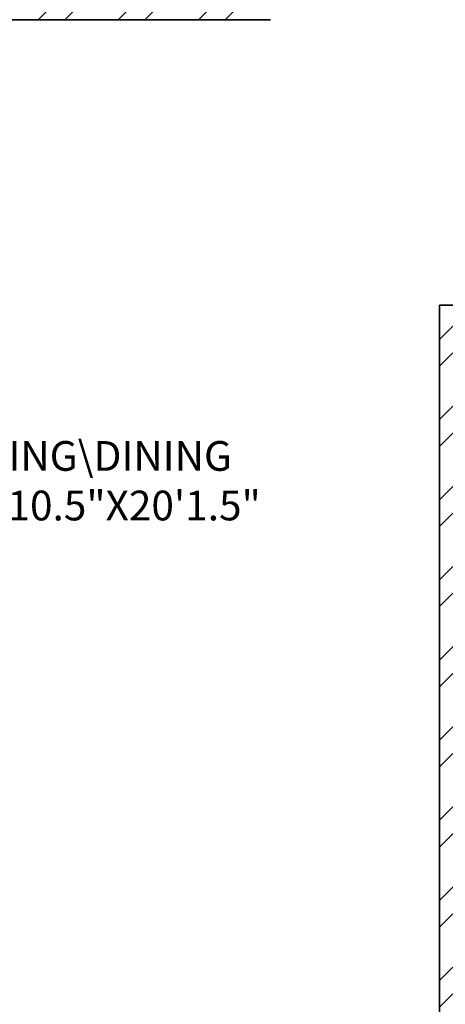
# Model space of a CAD drawing. Units: inches. Extents: x 2120 to 4013, y 1390 to 3019.
# Tile 38 of 59: x 2789 to 2861, y 2048 to 2213. Entities that reach past the tile are written whole.
import ezdxf

# ---------------------------------------------------------------- set-up
doc = ezdxf.new("R2010")
doc.units = ezdxf.units.IN
for name, color, linetype, lineweight in [('A-AREA-IDEN', 7, 'Continuous', 18), ('A-WALL', 7, 'Continuous', 35), ('A-WALL-PATT', 252, 'Continuous', 13)]:
    doc.layers.add(name, color=color, linetype=linetype, lineweight=lineweight)
doc.styles.get("Standard").update_dxf_attribs({"font": 'arial.ttf'})

msp = doc.modelspace()

# ---------------------------------------------------------------- hatches: boundary and pattern name
at = {"layer": 'A-WALL-PATT'}
h = msp.add_hatch(dxfattribs=at)
h.set_pattern_fill('ANSI32', color=256)
h.paths.add_polyline_path([(2271.7331, 2343.531), (2283.3788, 2343.531), (2283.3788, 2348.031), (2283.3788, 2352.5306), (2262.7331, 2352.5306), (2262.7331, 2182.638), (2267.2331, 2182.638), (2271.7331, 2182.638), (2271.7331, 2219.031), (2391.7331, 2219.031), (2391.7331, 2214.189), (2393.9831, 2214.189), (2396.2331, 2214.189), (2396.2331, 2219.031), (2420.2331, 2219.031), (2420.2331, 2225.7535), (2417.2197, 2225.7535), (2415.7331, 2225.7535), (2415.7331, 2223.5306), (2271.7331, 2223.5306)])
h.paths.add_polyline_path([(2380.0942, 2352.5306), (2343.3788, 2352.5306), (2343.3788, 2343.531), (2363.2331, 2343.531), (2363.2331, 2288.8489), (2365.4831, 2288.8489), (2367.7331, 2288.8489), (2367.7331, 2343.531), (2380.0942, 2343.531)], flags=17)
h.paths.add_polyline_path([(2432.4339, 2352.5306), (2404.0943, 2352.5306), (2404.0943, 2343.531), (2415.7331, 2343.531), (2415.7331, 2264.0306), (2367.7331, 2264.0306), (2367.7331, 2266.4872), (2363.2331, 2266.4872), (2363.2331, 2259.531), (2367.7331, 2259.531), (2415.7331, 2259.531), (2415.7331, 2255.0658), (2420.2331, 2255.0658), (2420.2331, 2259.531), (2424.5717, 2259.531), (2424.5717, 2261.781), (2424.5717, 2264.0306), (2420.2331, 2264.0306), (2420.2331, 2343.531), (2432.4339, 2343.531)])
h.paths.add_polyline_path([(2508.9115, 2352.5306), (2456.4339, 2352.5306), (2456.4339, 2343.531), (2468.2331, 2343.531), (2468.2331, 2264.0306), (2448.0487, 2264.0306), (2448.0487, 2259.531), (2468.2331, 2259.531), (2468.2331, 2255.5496), (2472.7331, 2255.5496), (2472.7331, 2343.531), (2508.9115, 2343.531)])
h.paths.add_polyline_path([(2637.7331, 2352.5306), (2544.9116, 2352.5306), (2544.9116, 2343.531), (2589.7331, 2343.531), (2633.2331, 2343.531), (2637.7331, 2343.531)])
h.paths.add_polyline_path([(2594.2331, 2343.5306), (2589.7331, 2343.5306), (2589.7331, 2259.5306), (2589.7331, 2252.4915), (2591.9831, 2252.4915), (2594.2331, 2252.4915)])
h.paths.add_polyline_path([(2637.7331, 2223.5306), (2594.2331, 2223.5306), (2594.2331, 2230.1988), (2591.9831, 2230.1988), (2589.7331, 2230.1988), (2589.7331, 2223.5306), (2472.7331, 2223.5306), (2468.2331, 2223.5306), (2468.2331, 2219.031), (2628.7331, 2219.031), (2628.7331, 2138.031), (2637.7331, 2138.031)])
h.paths.add_polyline_path([(3822.6535, 2458.4402), (3874.9468, 2458.4402), (3874.9468, 2476.9866), (3822.6535, 2476.9866)], flags=9)
h.paths.add_polyline_path([(3834.6921, 2781.8174), (3935.9206, 2781.8174), (3935.9206, 2800.3638), (3834.6921, 2800.3638)], flags=9)
h.paths.add_polyline_path([(3832.2843, 2837.9683), (3884.5776, 2837.9683), (3884.5776, 2856.5146), (3832.2843, 2856.5146)], flags=9)
h.paths.add_polyline_path([(3830.9388, 2861.4782), (3956.8958, 2861.4782), (3956.8958, 2880.0245), (3830.9388, 2880.0245)], flags=9)
h.paths.add_polyline_path([(3870.6966, 2352.5752), (3887.9272, 2352.5752), (3887.9272, 2377.3037), (3870.6966, 2377.3037)], flags=9)
h.paths.add_polyline_path([(3289.2701, 2413.161), (3435.2223, 2413.161), (3435.2223, 2450.2538), (3289.2701, 2450.2538)], flags=9)
h.paths.add_polyline_path([(2487.6944, 2414.3601), (2637.8335, 2414.3601), (2637.8335, 2451.4528), (2487.6944, 2451.4528)], flags=9)
h.paths.add_polyline_path([(2567.3724, 1457.9199), (2815.296, 1457.9199), (2815.296, 1495.0127), (2567.3724, 1495.0127)], flags=9)
h.paths.add_polyline_path([(2655.3825, 2093.2363), (2685.9555, 2093.2363), (2685.9555, 2111.8937), (2655.3825, 2111.8937)], flags=9)
h.paths.add_polyline_path([(2543.9218, 1550.6671), (2587.8406, 1550.6671), (2587.8406, 1569.3244), (2543.9218, 1569.3244)], flags=9)
h.paths.add_polyline_path([(2905.1384, 1543.8113), (2949.0572, 1543.8113), (2949.0572, 1562.4686), (2905.1384, 1562.4686)], flags=9)
h.paths.add_polyline_path([(2736.4118, 1702.4736), (2784.2153, 1702.4736), (2784.2153, 1721.1309), (2736.4118, 1721.1309)], flags=9)
h.paths.add_polyline_path([(2912.8666, 1710.4168), (2951.707, 1710.4168), (2951.707, 1729.0741), (2912.8666, 1729.0741)], flags=9)
h.paths.add_polyline_path([(2923.5785, 1763.5038), (2959.7279, 1763.5038), (2959.7279, 1782.1611), (2923.5785, 1782.1611)], flags=9)
h.paths.add_polyline_path([(2925.2114, 1809.6137), (2967.1861, 1809.6137), (2967.1861, 1828.271), (2925.2114, 1828.271)], flags=9)
h.paths.add_polyline_path([(2996.2711, 1878.9003), (2996.2711, 1913.109), (2977.6138, 1913.109), (2977.6138, 1878.9003)], flags=9)
h.paths.add_polyline_path([(2883.0859, 1895.7192), (2927.1855, 1895.7192), (2927.1855, 1914.3766), (2883.0859, 1914.3766)], flags=9)
h.paths.add_polyline_path([(2787.3924, 1810.8013), (2841.0213, 1810.8013), (2841.0213, 1829.4587), (2787.3924, 1829.4587)], flags=9)
h.paths.add_polyline_path([(2775.6399, 2101.7395), (2829.2689, 2101.7395), (2829.2689, 2120.3968), (2775.6399, 2120.3968)], flags=9)
h.paths.add_polyline_path([(2913.0263, 2075.817), (2951.8667, 2075.817), (2951.8667, 2094.4744), (2913.0263, 2094.4744)], flags=9)
h.paths.add_polyline_path([(2929.966, 2133.3669), (2966.1154, 2133.3669), (2966.1154, 2152.0243), (2929.966, 2152.0243)], flags=9)
h.paths.add_polyline_path([(2932.7502, 2182.6088), (2968.8996, 2182.6088), (2968.8996, 2201.2662), (2932.7502, 2201.2662)], flags=9)
h.paths.add_polyline_path([(2996.0681, 2266.3173), (2996.0681, 2300.5261), (2977.4108, 2300.5261), (2977.4108, 2266.3173)], flags=9)
h.paths.add_polyline_path([(2885.1039, 2279.2186), (2929.2035, 2279.2186), (2929.2035, 2297.8759), (2885.1039, 2297.8759)], flags=9)
h.paths.add_polyline_path([(2735.7042, 2218.3197), (2783.5078, 2218.3197), (2783.5078, 2236.9771), (2735.7042, 2236.9771)], flags=9)
h.paths.add_polyline_path([(2635.6049, 2044.0085), (2648.9678, 2044.0085), (2648.9678, 2054.312), (2635.6049, 2054.312)], flags=9)
h.paths.add_polyline_path([(2714.0148, 1923.0473), (2727.3777, 1923.0473), (2727.3777, 1933.3508), (2714.0148, 1933.3508)], flags=9)
h.paths.add_polyline_path([(2709.0345, 1988.1628), (2722.3974, 1988.1628), (2722.3974, 1998.4663), (2709.0345, 1998.4663)], flags=9)
h.paths.add_polyline_path([(2592.8935, 1962.1763), (2606.2564, 1962.1763), (2606.2564, 1972.4799), (2592.8935, 1972.4799)], flags=9)
h.paths.add_polyline_path([(2618.3996, 1985.9724), (2644.1942, 1985.9724), (2644.1942, 1996.2759), (2618.3996, 1996.2759)], flags=9)
h.paths.add_polyline_path([(2601.279, 1920.5869), (2614.6419, 1920.5869), (2614.6419, 1930.8904), (2601.279, 1930.8904)], flags=9)
h.paths.add_polyline_path([(2692.3278, 1932.7645), (2704.5311, 1932.7645), (2704.5311, 1943.0681), (2692.3278, 1943.0681)], flags=9)
h.paths.add_polyline_path([(2311.122, 1672.7318), (2355.0408, 1672.7318), (2355.0408, 1691.3892), (2311.122, 1691.3892)], flags=9)
h.paths.add_polyline_path([(2456.2551, 1632.3198), (2492.4796, 1632.3198), (2492.4796, 1650.9772), (2456.2551, 1650.9772)], flags=9)
h.paths.add_polyline_path([(2401.0766, 1631.4793), (2437.301, 1631.4793), (2437.301, 1650.1367), (2401.0766, 1650.1367)], flags=9)
h.paths.add_polyline_path([(2546.7054, 1700.9235), (2594.509, 1700.9235), (2594.509, 1719.5809), (2546.7054, 1719.5809)], flags=9)
h.paths.add_polyline_path([(2445.4866, 1766.9937), (2497.5261, 1766.9937), (2497.5261, 1785.651), (2445.4866, 1785.651)], flags=9)
h.paths.add_polyline_path([(2287.9992, 1739.7675), (2326.8396, 1739.7675), (2326.8396, 1758.4248), (2287.9992, 1758.4248)], flags=9)
h.paths.add_polyline_path([(2458.5279, 1924.7607), (2510.5675, 1924.7607), (2510.5675, 1943.4181), (2458.5279, 1943.4181)], flags=9)
h.paths.add_polyline_path([(2309.2811, 1902.7642), (2345.4305, 1902.7642), (2345.4305, 1921.4215), (2309.2811, 1921.4215)], flags=9)
h.paths.add_polyline_path([(2490.7554, 2018.9392), (2530.7896, 2018.9392), (2530.7896, 2037.5965), (2490.7554, 2037.5965)], flags=9)
h.paths.add_polyline_path([(2402.143, 2024.7393), (2438.5414, 2024.7393), (2438.5414, 2043.3966), (2402.143, 2043.3966)], flags=9)
h.paths.add_polyline_path([(2287.856, 1931.7926), (2326.6964, 1931.7926), (2326.6964, 1950.4499), (2287.856, 1950.4499)], flags=9)
h.paths.add_polyline_path([(2281.7979, 2193.5771), (2320.6383, 2193.5771), (2320.6383, 2212.2344), (2281.7979, 2212.2344)], flags=25)
h.paths.add_polyline_path([(2484.0754, 2093.892), (2536.115, 2093.892), (2536.115, 2112.5494), (2484.0754, 2112.5494)], flags=9)
h.paths.add_polyline_path([(2624.7948, 2281.8639), (2624.7948, 2311.4137), (2606.1375, 2311.4137), (2606.1375, 2281.8639)], flags=9)
h.paths.add_polyline_path([(2507.5036, 2290.3639), (2541.934, 2290.3639), (2541.934, 2309.0212), (2507.5036, 2309.0212)], flags=9)
h.paths.add_polyline_path([(2423.1076, 2285.2202), (2459.332, 2285.2202), (2459.332, 2303.8776), (2423.1076, 2303.8776)], flags=9)
h.paths.add_polyline_path([(2374.5467, 2289.6272), (2410.7711, 2289.6272), (2410.7711, 2308.2846), (2374.5467, 2308.2846)], flags=25)
h.paths.add_polyline_path([(2277.4907, 2227.5651), (2316.3311, 2227.5651), (2316.3311, 2246.2224), (2277.4907, 2246.2224)], flags=25)
h.paths.add_polyline_path([(2655.3825, 2093.2367), (2685.9555, 2093.2367), (2685.9555, 2111.894), (2655.3825, 2111.894)], flags=9)
h.paths.add_polyline_path([(2543.9217, 1550.6674), (2587.8406, 1550.6674), (2587.8406, 1569.3247), (2543.9217, 1569.3247)], flags=9)
h.paths.add_polyline_path([(2905.1384, 1543.8116), (2949.0572, 1543.8116), (2949.0572, 1562.4689), (2905.1384, 1562.4689)], flags=9)
h.paths.add_polyline_path([(2736.4118, 1702.4739), (2784.2153, 1702.4739), (2784.2153, 1721.1312), (2736.4118, 1721.1312)], flags=9)
h.paths.add_polyline_path([(2912.8666, 1710.4171), (2951.707, 1710.4171), (2951.707, 1729.0744), (2912.8666, 1729.0744)], flags=9)
h.paths.add_polyline_path([(2923.5785, 1763.5041), (2959.7279, 1763.5041), (2959.7279, 1782.1614), (2923.5785, 1782.1614)], flags=9)
h.paths.add_polyline_path([(2925.2114, 1809.614), (2967.1861, 1809.614), (2967.1861, 1828.2713), (2925.2114, 1828.2713)], flags=9)
h.paths.add_polyline_path([(2996.2711, 1878.9006), (2996.2711, 1913.1094), (2977.6137, 1913.1094), (2977.6137, 1878.9006)], flags=9)
h.paths.add_polyline_path([(2883.0859, 1895.7195), (2927.1855, 1895.7195), (2927.1855, 1914.3769), (2883.0859, 1914.3769)], flags=9)
h.paths.add_polyline_path([(2787.3924, 1810.8016), (2841.0213, 1810.8016), (2841.0213, 1829.459), (2787.3924, 1829.459)], flags=9)
h.paths.add_polyline_path([(2775.6399, 2101.7398), (2829.2688, 2101.7398), (2829.2688, 2120.3971), (2775.6399, 2120.3971)], flags=9)
h.paths.add_polyline_path([(2913.0263, 2075.8173), (2951.8667, 2075.8173), (2951.8667, 2094.4747), (2913.0263, 2094.4747)], flags=9)
h.paths.add_polyline_path([(2929.966, 2133.3672), (2966.1154, 2133.3672), (2966.1154, 2152.0246), (2929.966, 2152.0246)], flags=9)
h.paths.add_polyline_path([(2932.7502, 2182.6091), (2968.8996, 2182.6091), (2968.8996, 2201.2665), (2932.7502, 2201.2665)], flags=9)
h.paths.add_polyline_path([(2996.0681, 2266.3176), (2996.0681, 2300.5264), (2977.4108, 2300.5264), (2977.4108, 2266.3176)], flags=9)
h.paths.add_polyline_path([(2885.1039, 2279.2189), (2929.2035, 2279.2189), (2929.2035, 2297.8762), (2885.1039, 2297.8762)], flags=9)
h.paths.add_polyline_path([(2735.7042, 2218.32), (2783.5078, 2218.32), (2783.5078, 2236.9774), (2735.7042, 2236.9774)], flags=9)
h.paths.add_polyline_path([(2635.6048, 2044.0088), (2648.9677, 2044.0088), (2648.9677, 2054.3123), (2635.6048, 2054.3123)], flags=9)
h.paths.add_polyline_path([(2714.0148, 1923.0476), (2727.3777, 1923.0476), (2727.3777, 1933.3511), (2714.0148, 1933.3511)], flags=9)
h.paths.add_polyline_path([(2709.0345, 1988.1631), (2722.3974, 1988.1631), (2722.3974, 1998.4666), (2709.0345, 1998.4666)], flags=9)
h.paths.add_polyline_path([(2592.8935, 1962.1766), (2606.2564, 1962.1766), (2606.2564, 1972.4802), (2592.8935, 1972.4802)], flags=9)
h.paths.add_polyline_path([(2618.3995, 1985.9727), (2644.1942, 1985.9727), (2644.1942, 1996.2762), (2618.3995, 1996.2762)], flags=9)
h.paths.add_polyline_path([(2601.279, 1920.5872), (2614.6419, 1920.5872), (2614.6419, 1930.8908), (2601.279, 1930.8908)], flags=9)
h.paths.add_polyline_path([(2692.3278, 1932.7648), (2704.5311, 1932.7648), (2704.5311, 1943.0684), (2692.3278, 1943.0684)], flags=9)
h.paths.add_polyline_path([(2311.122, 1672.7321), (2355.0408, 1672.7321), (2355.0408, 1691.3895), (2311.122, 1691.3895)], flags=9)
h.paths.add_polyline_path([(2456.2551, 1632.3201), (2492.4795, 1632.3201), (2492.4795, 1650.9775), (2456.2551, 1650.9775)], flags=9)
h.paths.add_polyline_path([(2401.0766, 1631.4796), (2437.301, 1631.4796), (2437.301, 1650.137), (2401.0766, 1650.137)], flags=9)
h.paths.add_polyline_path([(2546.7054, 1700.9238), (2594.509, 1700.9238), (2594.509, 1719.5812), (2546.7054, 1719.5812)], flags=9)
h.paths.add_polyline_path([(2445.4866, 1766.994), (2497.5261, 1766.994), (2497.5261, 1785.6513), (2445.4866, 1785.6513)], flags=9)
h.paths.add_polyline_path([(2287.9992, 1739.7678), (2326.8396, 1739.7678), (2326.8396, 1758.4251), (2287.9992, 1758.4251)], flags=9)
h.paths.add_polyline_path([(2458.5279, 1924.7611), (2510.5675, 1924.7611), (2510.5675, 1943.4184), (2458.5279, 1943.4184)], flags=9)
h.paths.add_polyline_path([(2309.2811, 1902.7645), (2345.4305, 1902.7645), (2345.4305, 1921.4218), (2309.2811, 1921.4218)], flags=9)
h.paths.add_polyline_path([(2490.7554, 2018.9395), (2530.7895, 2018.9395), (2530.7895, 2037.5968), (2490.7554, 2037.5968)], flags=9)
h.paths.add_polyline_path([(2402.143, 2024.7396), (2438.5413, 2024.7396), (2438.5413, 2043.3969), (2402.143, 2043.3969)], flags=9)
h.paths.add_polyline_path([(2287.856, 1931.7929), (2326.6964, 1931.7929), (2326.6964, 1950.4502), (2287.856, 1950.4502)], flags=9)
h.paths.add_polyline_path([(2281.7979, 2193.5774), (2320.6383, 2193.5774), (2320.6383, 2212.2347), (2281.7979, 2212.2347)], flags=25)
h.paths.add_polyline_path([(2484.0754, 2093.8924), (2536.115, 2093.8924), (2536.115, 2112.5497), (2484.0754, 2112.5497)], flags=9)
h.paths.add_polyline_path([(2624.7948, 2281.8642), (2624.7948, 2311.414), (2606.1374, 2311.414), (2606.1374, 2281.8642)], flags=9)
h.paths.add_polyline_path([(2507.5035, 2290.3642), (2541.934, 2290.3642), (2541.934, 2309.0215), (2507.5035, 2309.0215)], flags=9)
h.paths.add_polyline_path([(2423.1075, 2285.2205), (2459.332, 2285.2205), (2459.332, 2303.8779), (2423.1075, 2303.8779)], flags=9)
h.paths.add_polyline_path([(2374.5467, 2289.6275), (2410.7711, 2289.6275), (2410.7711, 2308.2849), (2374.5467, 2308.2849)], flags=25)
h.paths.add_polyline_path([(2277.4907, 2227.5654), (2316.3311, 2227.5654), (2316.3311, 2246.2227), (2277.4907, 2246.2227)], flags=25)
h = msp.add_hatch(dxfattribs=at)
h.set_pattern_fill('ANSI32', color=256)
h.paths.add_polyline_path([(2271.7331, 1980.389), (2262.7331, 1980.389), (2262.7331, 1912.8434), (2267.2331, 1912.8434), (2271.7331, 1912.8434), (2271.7331, 1922.531), (2351.2331, 1922.531), (2351.2331, 1901.4728), (2355.7331, 1901.4728), (2355.7331, 1922.531), (2357.9815, 1922.531), (2357.9815, 1926.5306), (2271.7331, 1926.5306)])
h.paths.add_polyline_path([(2589.2331, 1949.1622), (2584.7331, 1949.1622), (2580.2331, 1949.1622), (2580.2331, 1874.5306), (2355.7331, 1874.5306), (2355.7331, 1880.1922), (2351.2331, 1880.1922), (2351.2331, 1874.5306), (2271.7331, 1874.5306), (2271.7331, 1888.8431), (2262.7331, 1888.8431), (2262.7331, 1842.2909), (2267.2331, 1842.2909), (2271.7331, 1842.2909), (2271.7331, 1865.531), (2415.7331, 1865.531), (2415.7331, 1779.7286), (2420.2331, 1779.7286), (2420.2331, 1865.531), (2589.2331, 1865.531)])
h.paths.add_polyline_path([(2271.7331, 1782.2906), (2262.7331, 1782.2906), (2262.7331, 1711.4639), (2267.2331, 1711.4639), (2271.7331, 1711.4639), (2271.7331, 1738.031), (2420.2331, 1738.031), (2420.2331, 1742.531), (2420.2331, 1747.3376), (2417.9831, 1747.3376), (2415.7331, 1747.3376), (2415.7331, 1742.5306), (2271.7331, 1742.5306)])
h.paths.add_polyline_path([(2271.7331, 1627.031), (2362.3957, 1627.031), (2362.3957, 1629.281), (2362.3957, 1631.5306), (2271.7331, 1631.5306), (2271.7331, 1675.4636), (2262.7331, 1675.4636), (2262.7331, 1581.531), (2405.3032, 1581.531), (2405.3032, 1586.031), (2405.3032, 1590.5306), (2396.2331, 1590.5306), (2396.2331, 1691.4513), (2418.7206, 1691.4513), (2418.7206, 1695.951), (2396.2331, 1695.951), (2391.7331, 1695.951), (2391.7331, 1631.5306), (2386.7425, 1631.5306), (2386.7425, 1629.2806), (2386.7425, 1627.031), (2391.7331, 1627.031), (2391.7331, 1586.1709), (2271.7331, 1586.1709)])
h.paths.add_polyline_path([(2459.6703, 1590.5306), (2429.3032, 1590.5306), (2429.3032, 1581.531), (2459.6703, 1581.531), (2459.6703, 1586.031)])
h.paths.add_polyline_path([(2501.2331, 1590.531), (2501.2331, 1665.0195), (2498.9831, 1665.0195), (2496.7331, 1665.0195), (2496.7331, 1590.5306), (2483.8201, 1590.5306), (2483.8201, 1590.1579), (2483.6704, 1590.1579), (2483.6704, 1581.531), (2505.0196, 1581.531), (2505.0196, 1583.781), (2505.0196, 1586.0306), (2501.2331, 1586.0306)])
h.paths.add_polyline_path([(2544.1361, 1583.781), (2544.1361, 1586.0306), (2527.1368, 1586.0306), (2527.1368, 1583.7806), (2527.1368, 1581.531), (2544.1361, 1581.531)])
h.paths.add_polyline_path([(3822.6535, 2458.4402), (3874.9468, 2458.4402), (3874.9468, 2476.9866), (3822.6535, 2476.9866)], flags=9)
h.paths.add_polyline_path([(3834.6921, 2781.8174), (3935.9206, 2781.8174), (3935.9206, 2800.3638), (3834.6921, 2800.3638)], flags=9)
h.paths.add_polyline_path([(3832.2843, 2837.9683), (3884.5776, 2837.9683), (3884.5776, 2856.5146), (3832.2843, 2856.5146)], flags=9)
h.paths.add_polyline_path([(3830.9388, 2861.4782), (3956.8958, 2861.4782), (3956.8958, 2880.0245), (3830.9388, 2880.0245)], flags=9)
h.paths.add_polyline_path([(3870.6966, 2352.5752), (3887.9272, 2352.5752), (3887.9272, 2377.3037), (3870.6966, 2377.3037)], flags=9)
h.paths.add_polyline_path([(3289.2701, 2413.161), (3435.2223, 2413.161), (3435.2223, 2450.2538), (3289.2701, 2450.2538)], flags=9)
h.paths.add_polyline_path([(2487.6944, 2414.3601), (2637.8335, 2414.3601), (2637.8335, 2451.4528), (2487.6944, 2451.4528)], flags=9)
h.paths.add_polyline_path([(2567.3724, 1457.9199), (2815.296, 1457.9199), (2815.296, 1495.0127), (2567.3724, 1495.0127)], flags=9)
h.paths.add_polyline_path([(2655.3825, 2093.2363), (2685.9555, 2093.2363), (2685.9555, 2111.8937), (2655.3825, 2111.8937)], flags=9)
h.paths.add_polyline_path([(2543.9218, 1550.6671), (2587.8406, 1550.6671), (2587.8406, 1569.3244), (2543.9218, 1569.3244)], flags=9)
h.paths.add_polyline_path([(2905.1384, 1543.8113), (2949.0572, 1543.8113), (2949.0572, 1562.4686), (2905.1384, 1562.4686)], flags=9)
h.paths.add_polyline_path([(2736.4118, 1702.4736), (2784.2153, 1702.4736), (2784.2153, 1721.1309), (2736.4118, 1721.1309)], flags=9)
h.paths.add_polyline_path([(2912.8666, 1710.4168), (2951.707, 1710.4168), (2951.707, 1729.0741), (2912.8666, 1729.0741)], flags=9)
h.paths.add_polyline_path([(2923.5785, 1763.5038), (2959.7279, 1763.5038), (2959.7279, 1782.1611), (2923.5785, 1782.1611)], flags=9)
h.paths.add_polyline_path([(2925.2114, 1809.6137), (2967.1861, 1809.6137), (2967.1861, 1828.271), (2925.2114, 1828.271)], flags=9)
h.paths.add_polyline_path([(2996.2711, 1878.9003), (2996.2711, 1913.109), (2977.6138, 1913.109), (2977.6138, 1878.9003)], flags=9)
h.paths.add_polyline_path([(2883.0859, 1895.7192), (2927.1855, 1895.7192), (2927.1855, 1914.3766), (2883.0859, 1914.3766)], flags=9)
h.paths.add_polyline_path([(2787.3924, 1810.8013), (2841.0213, 1810.8013), (2841.0213, 1829.4587), (2787.3924, 1829.4587)], flags=9)
h.paths.add_polyline_path([(2775.6399, 2101.7395), (2829.2689, 2101.7395), (2829.2689, 2120.3968), (2775.6399, 2120.3968)], flags=9)
h.paths.add_polyline_path([(2913.0263, 2075.817), (2951.8667, 2075.817), (2951.8667, 2094.4744), (2913.0263, 2094.4744)], flags=9)
h.paths.add_polyline_path([(2929.966, 2133.3669), (2966.1154, 2133.3669), (2966.1154, 2152.0243), (2929.966, 2152.0243)], flags=9)
h.paths.add_polyline_path([(2932.7502, 2182.6088), (2968.8996, 2182.6088), (2968.8996, 2201.2662), (2932.7502, 2201.2662)], flags=9)
h.paths.add_polyline_path([(2996.0681, 2266.3173), (2996.0681, 2300.5261), (2977.4108, 2300.5261), (2977.4108, 2266.3173)], flags=9)
h.paths.add_polyline_path([(2885.1039, 2279.2186), (2929.2035, 2279.2186), (2929.2035, 2297.8759), (2885.1039, 2297.8759)], flags=9)
h.paths.add_polyline_path([(2735.7042, 2218.3197), (2783.5078, 2218.3197), (2783.5078, 2236.9771), (2735.7042, 2236.9771)], flags=9)
h.paths.add_polyline_path([(2635.6049, 2044.0085), (2648.9678, 2044.0085), (2648.9678, 2054.312), (2635.6049, 2054.312)], flags=9)
h.paths.add_polyline_path([(2714.0148, 1923.0473), (2727.3777, 1923.0473), (2727.3777, 1933.3508), (2714.0148, 1933.3508)], flags=9)
h.paths.add_polyline_path([(2709.0345, 1988.1628), (2722.3974, 1988.1628), (2722.3974, 1998.4663), (2709.0345, 1998.4663)], flags=9)
h.paths.add_polyline_path([(2592.8935, 1962.1763), (2606.2564, 1962.1763), (2606.2564, 1972.4799), (2592.8935, 1972.4799)], flags=9)
h.paths.add_polyline_path([(2618.3996, 1985.9724), (2644.1942, 1985.9724), (2644.1942, 1996.2759), (2618.3996, 1996.2759)], flags=9)
h.paths.add_polyline_path([(2601.279, 1920.5869), (2614.6419, 1920.5869), (2614.6419, 1930.8904), (2601.279, 1930.8904)], flags=9)
h.paths.add_polyline_path([(2692.3278, 1932.7645), (2704.5311, 1932.7645), (2704.5311, 1943.0681), (2692.3278, 1943.0681)], flags=9)
h.paths.add_polyline_path([(2311.122, 1672.7318), (2355.0408, 1672.7318), (2355.0408, 1691.3892), (2311.122, 1691.3892)], flags=25)
h.paths.add_polyline_path([(2456.2551, 1632.3198), (2492.4796, 1632.3198), (2492.4796, 1650.9772), (2456.2551, 1650.9772)], flags=9)
h.paths.add_polyline_path([(2401.0766, 1631.4793), (2437.301, 1631.4793), (2437.301, 1650.1367), (2401.0766, 1650.1367)], flags=9)
h.paths.add_polyline_path([(2546.7054, 1700.9235), (2594.509, 1700.9235), (2594.509, 1719.5809), (2546.7054, 1719.5809)], flags=9)
h.paths.add_polyline_path([(2445.4866, 1766.9937), (2497.5261, 1766.9937), (2497.5261, 1785.651), (2445.4866, 1785.651)], flags=9)
h.paths.add_polyline_path([(2287.9992, 1739.7675), (2326.8396, 1739.7675), (2326.8396, 1758.4248), (2287.9992, 1758.4248)], flags=24)
h.paths.add_polyline_path([(2458.5279, 1924.7607), (2510.5675, 1924.7607), (2510.5675, 1943.4181), (2458.5279, 1943.4181)], flags=25)
h.paths.add_polyline_path([(2309.2811, 1902.7642), (2345.4305, 1902.7642), (2345.4305, 1921.4215), (2309.2811, 1921.4215)], flags=25)
h.paths.add_polyline_path([(2490.7554, 2018.9392), (2530.7896, 2018.9392), (2530.7896, 2037.5965), (2490.7554, 2037.5965)], flags=9)
h.paths.add_polyline_path([(2402.143, 2024.7393), (2438.5414, 2024.7393), (2438.5414, 2043.3966), (2402.143, 2043.3966)], flags=9)
h.paths.add_polyline_path([(2287.856, 1931.7926), (2326.6964, 1931.7926), (2326.6964, 1950.4499), (2287.856, 1950.4499)], flags=25)
h.paths.add_polyline_path([(2281.7979, 2193.5771), (2320.6383, 2193.5771), (2320.6383, 2212.2344), (2281.7979, 2212.2344)], flags=9)
h.paths.add_polyline_path([(2484.0754, 2093.892), (2536.115, 2093.892), (2536.115, 2112.5494), (2484.0754, 2112.5494)], flags=9)
h.paths.add_polyline_path([(2624.7948, 2281.8639), (2624.7948, 2311.4137), (2606.1375, 2311.4137), (2606.1375, 2281.8639)], flags=9)
h.paths.add_polyline_path([(2507.5036, 2290.3639), (2541.934, 2290.3639), (2541.934, 2309.0212), (2507.5036, 2309.0212)], flags=9)
h.paths.add_polyline_path([(2423.1076, 2285.2202), (2459.332, 2285.2202), (2459.332, 2303.8776), (2423.1076, 2303.8776)], flags=9)
h.paths.add_polyline_path([(2374.5467, 2289.6272), (2410.7711, 2289.6272), (2410.7711, 2308.2846), (2374.5467, 2308.2846)], flags=9)
h.paths.add_polyline_path([(2277.4907, 2227.5651), (2316.3311, 2227.5651), (2316.3311, 2246.2224), (2277.4907, 2246.2224)], flags=9)
h.paths.add_polyline_path([(2655.3825, 2093.2367), (2685.9555, 2093.2367), (2685.9555, 2111.894), (2655.3825, 2111.894)], flags=9)
h.paths.add_polyline_path([(2543.9217, 1550.6674), (2587.8406, 1550.6674), (2587.8406, 1569.3247), (2543.9217, 1569.3247)], flags=9)
h.paths.add_polyline_path([(2905.1384, 1543.8116), (2949.0572, 1543.8116), (2949.0572, 1562.4689), (2905.1384, 1562.4689)], flags=9)
h.paths.add_polyline_path([(2736.4118, 1702.4739), (2784.2153, 1702.4739), (2784.2153, 1721.1312), (2736.4118, 1721.1312)], flags=9)
h.paths.add_polyline_path([(2912.8666, 1710.4171), (2951.707, 1710.4171), (2951.707, 1729.0744), (2912.8666, 1729.0744)], flags=9)
h.paths.add_polyline_path([(2923.5785, 1763.5041), (2959.7279, 1763.5041), (2959.7279, 1782.1614), (2923.5785, 1782.1614)], flags=9)
h.paths.add_polyline_path([(2925.2114, 1809.614), (2967.1861, 1809.614), (2967.1861, 1828.2713), (2925.2114, 1828.2713)], flags=9)
h.paths.add_polyline_path([(2996.2711, 1878.9006), (2996.2711, 1913.1094), (2977.6137, 1913.1094), (2977.6137, 1878.9006)], flags=9)
h.paths.add_polyline_path([(2883.0859, 1895.7195), (2927.1855, 1895.7195), (2927.1855, 1914.3769), (2883.0859, 1914.3769)], flags=9)
h.paths.add_polyline_path([(2787.3924, 1810.8016), (2841.0213, 1810.8016), (2841.0213, 1829.459), (2787.3924, 1829.459)], flags=9)
h.paths.add_polyline_path([(2775.6399, 2101.7398), (2829.2688, 2101.7398), (2829.2688, 2120.3971), (2775.6399, 2120.3971)], flags=9)
h.paths.add_polyline_path([(2913.0263, 2075.8173), (2951.8667, 2075.8173), (2951.8667, 2094.4747), (2913.0263, 2094.4747)], flags=9)
h.paths.add_polyline_path([(2929.966, 2133.3672), (2966.1154, 2133.3672), (2966.1154, 2152.0246), (2929.966, 2152.0246)], flags=9)
h.paths.add_polyline_path([(2932.7502, 2182.6091), (2968.8996, 2182.6091), (2968.8996, 2201.2665), (2932.7502, 2201.2665)], flags=9)
h.paths.add_polyline_path([(2996.0681, 2266.3176), (2996.0681, 2300.5264), (2977.4108, 2300.5264), (2977.4108, 2266.3176)], flags=9)
h.paths.add_polyline_path([(2885.1039, 2279.2189), (2929.2035, 2279.2189), (2929.2035, 2297.8762), (2885.1039, 2297.8762)], flags=9)
h.paths.add_polyline_path([(2735.7042, 2218.32), (2783.5078, 2218.32), (2783.5078, 2236.9774), (2735.7042, 2236.9774)], flags=9)
h.paths.add_polyline_path([(2635.6048, 2044.0088), (2648.9677, 2044.0088), (2648.9677, 2054.3123), (2635.6048, 2054.3123)], flags=9)
h.paths.add_polyline_path([(2714.0148, 1923.0476), (2727.3777, 1923.0476), (2727.3777, 1933.3511), (2714.0148, 1933.3511)], flags=9)
h.paths.add_polyline_path([(2709.0345, 1988.1631), (2722.3974, 1988.1631), (2722.3974, 1998.4666), (2709.0345, 1998.4666)], flags=9)
h.paths.add_polyline_path([(2592.8935, 1962.1766), (2606.2564, 1962.1766), (2606.2564, 1972.4802), (2592.8935, 1972.4802)], flags=9)
h.paths.add_polyline_path([(2618.3995, 1985.9727), (2644.1942, 1985.9727), (2644.1942, 1996.2762), (2618.3995, 1996.2762)], flags=9)
h.paths.add_polyline_path([(2601.279, 1920.5872), (2614.6419, 1920.5872), (2614.6419, 1930.8908), (2601.279, 1930.8908)], flags=9)
h.paths.add_polyline_path([(2692.3278, 1932.7648), (2704.5311, 1932.7648), (2704.5311, 1943.0684), (2692.3278, 1943.0684)], flags=9)
h.paths.add_polyline_path([(2311.122, 1672.7321), (2355.0408, 1672.7321), (2355.0408, 1691.3895), (2311.122, 1691.3895)], flags=25)
h.paths.add_polyline_path([(2456.2551, 1632.3201), (2492.4795, 1632.3201), (2492.4795, 1650.9775), (2456.2551, 1650.9775)], flags=9)
h.paths.add_polyline_path([(2401.0766, 1631.4796), (2437.301, 1631.4796), (2437.301, 1650.137), (2401.0766, 1650.137)], flags=9)
h.paths.add_polyline_path([(2546.7054, 1700.9238), (2594.509, 1700.9238), (2594.509, 1719.5812), (2546.7054, 1719.5812)], flags=9)
h.paths.add_polyline_path([(2445.4866, 1766.994), (2497.5261, 1766.994), (2497.5261, 1785.6513), (2445.4866, 1785.6513)], flags=9)
h.paths.add_polyline_path([(2287.9992, 1739.7678), (2326.8396, 1739.7678), (2326.8396, 1758.4251), (2287.9992, 1758.4251)], flags=24)
h.paths.add_polyline_path([(2458.5279, 1924.7611), (2510.5675, 1924.7611), (2510.5675, 1943.4184), (2458.5279, 1943.4184)], flags=25)
h.paths.add_polyline_path([(2309.2811, 1902.7645), (2345.4305, 1902.7645), (2345.4305, 1921.4218), (2309.2811, 1921.4218)], flags=25)
h.paths.add_polyline_path([(2490.7554, 2018.9395), (2530.7895, 2018.9395), (2530.7895, 2037.5968), (2490.7554, 2037.5968)], flags=9)
h.paths.add_polyline_path([(2402.143, 2024.7396), (2438.5413, 2024.7396), (2438.5413, 2043.3969), (2402.143, 2043.3969)], flags=9)
h.paths.add_polyline_path([(2287.856, 1931.7929), (2326.6964, 1931.7929), (2326.6964, 1950.4502), (2287.856, 1950.4502)], flags=25)
h.paths.add_polyline_path([(2281.7979, 2193.5774), (2320.6383, 2193.5774), (2320.6383, 2212.2347), (2281.7979, 2212.2347)], flags=9)
h.paths.add_polyline_path([(2484.0754, 2093.8924), (2536.115, 2093.8924), (2536.115, 2112.5497), (2484.0754, 2112.5497)], flags=9)
h.paths.add_polyline_path([(2624.7948, 2281.8642), (2624.7948, 2311.414), (2606.1374, 2311.414), (2606.1374, 2281.8642)], flags=9)
h.paths.add_polyline_path([(2507.5035, 2290.3642), (2541.934, 2290.3642), (2541.934, 2309.0215), (2507.5035, 2309.0215)], flags=9)
h.paths.add_polyline_path([(2423.1075, 2285.2205), (2459.332, 2285.2205), (2459.332, 2303.8779), (2423.1075, 2303.8779)], flags=9)
h.paths.add_polyline_path([(2374.5467, 2289.6275), (2410.7711, 2289.6275), (2410.7711, 2308.2849), (2374.5467, 2308.2849)], flags=9)
h.paths.add_polyline_path([(2277.4907, 2227.5654), (2316.3311, 2227.5654), (2316.3311, 2246.2227), (2277.4907, 2246.2227)], flags=9)
h = msp.add_hatch(dxfattribs=at)
h.set_pattern_fill('ANSI32', color=256)
h.paths.add_polyline_path([(2271.7331, 2122.6377), (2262.7331, 2122.6377), (2262.7331, 2040.3893), (2267.2331, 2040.3893), (2271.7331, 2040.3893), (2271.7331, 2044.8856), (2271.7331, 2070.531), (2391.7331, 2070.531), (2391.7331, 1926.5306), (2388.3993, 1926.5306), (2388.3993, 1922.531), (2395.7331, 1922.531), (2395.7331, 1992.531), (2400.4511, 1992.531), (2400.4511, 1997.0306), (2395.7331, 1997.0306), (2395.7331, 2070.531), (2443.7331, 2070.531), (2443.7331, 2046.1368), (2448.2331, 2046.1368), (2448.2331, 2070.531), (2580.2331, 2070.531), (2580.2331, 1997.0306), (2492.9076, 1997.0306), (2492.9076, 1992.531), (2580.2331, 1992.531), (2580.2331, 1983.9368), (2589.2331, 1983.9368), (2589.2331, 2070.531), (2589.2331, 2075.0306), (2396.2331, 2075.0306), (2396.2331, 2184.3565), (2393.9831, 2184.3565), (2391.7331, 2184.3565), (2391.7331, 2075.0306), (2271.7331, 2075.0306)])
h.paths.add_polyline_path([(2724.7331, 2138.0306), (2628.7331, 2138.0306), (2628.7331, 2070.5306), (2628.7331, 2067.0987), (2633.2331, 2067.0987), (2637.7331, 2067.0987), (2637.7331, 2070.531), (2657.3413, 2070.531), (2657.3413, 2079.5306), (2637.7331, 2079.5306), (2637.7331, 2129.031), (2715.7331, 2129.031), (2715.7331, 2079.5306), (2698.0378, 2079.5306), (2698.0378, 2070.531), (2715.7331, 2070.531), (2715.7331, 2012.1531), (2720.2331, 2012.1531), (2724.7331, 2012.1531)])
h.paths.add_polyline_path([(2724.7331, 2213.031), (2831.3209, 2213.031), (2831.3209, 2215.281), (2831.3209, 2217.5306), (2724.7331, 2217.5306), (2724.7331, 2343.531), (2751.8755, 2343.531), (2751.8755, 2352.5306), (2715.7331, 2352.5306), (2715.7331, 2138.031), (2724.7331, 2138.031)])
h.paths.add_polyline_path([(2902.53, 2352.5306), (2811.8755, 2352.5306), (2811.8755, 2343.531), (2867.2331, 2343.531), (2867.2331, 2217.5306), (2863.6364, 2217.5306), (2863.6364, 2213.031), (2871.7331, 2213.031), (2871.7331, 2217.531), (2871.7331, 2343.531), (2902.53, 2343.531)])
h.paths.add_polyline_path([(3009.7331, 2352.5306), (2938.53, 2352.5306), (2938.53, 2343.531), (2966.2331, 2343.531), (2966.2331, 2242.3281), (2968.4831, 2242.3281), (2970.7331, 2242.3281), (2970.7331, 2343.531), (3009.7331, 2343.531)])
h.paths.add_polyline_path([(3009.7331, 2217.5306), (2970.7331, 2217.5306), (2970.7331, 2220.5422), (2968.4831, 2220.5422), (2966.2331, 2220.5422), (2966.2331, 2217.5306), (2911.7752, 2217.5306), (2907.7331, 2217.5306), (2907.7331, 2213.0306), (2907.7331, 2194.9663), (2912.2331, 2194.9663), (2912.2331, 2213.031), (2970.7331, 2213.031), (3000.7331, 2213.031), (3000.7331, 2205.523), (3009.7331, 2205.523)])
h.paths.add_polyline_path([(3009.7331, 2181.5227), (3000.7331, 2181.5227), (3000.7331, 2165.0306), (2912.2331, 2165.0306), (2912.2331, 2170.8202), (2907.7331, 2170.8202), (2907.7331, 2165.0306), (2899.5169, 2165.0306), (2899.5169, 2162.7806), (2899.5169, 2160.531), (2907.7331, 2160.531), (2907.7331, 2137.3432), (2912.2331, 2137.3432), (2912.2331, 2160.531), (3000.7331, 2160.531), (3000.7331, 2150.4993), (3009.7331, 2150.4993)])
h.paths.add_polyline_path([(3009.7331, 2126.499), (3005.2331, 2126.499), (3000.7331, 2126.499), (3000.7331, 2112.5306), (2912.2331, 2112.5306), (2912.2331, 2115.6036), (2907.7331, 2115.6036), (2907.7331, 2108.031), (3000.7331, 2108.031), (3000.7331, 2084.7256), (3009.7331, 2084.7256)], flags=17)
h.paths.add_polyline_path([(3009.7331, 1971.531), (3009.7331, 2024.7253), (3000.7331, 2024.7253), (3000.7331, 2006.4153), (3000.7331, 1971.5306), (2864.2331, 1971.5306), (2864.2331, 2160.531), (2868.0522, 2160.531), (2868.0522, 2165.0306), (2859.7331, 2165.0306), (2859.7331, 1971.5306), (2724.7331, 1971.5306), (2724.7331, 1977.7012), (2715.7331, 1977.7012), (2715.7331, 1962.5306), (2715.7331, 1950.9035), (2720.2331, 1950.9035), (2724.7331, 1950.9035), (2724.7331, 1962.531), (2855.2331, 1962.531), (2859.7331, 1962.531), (2859.7331, 1835.031), (2864.2331, 1834.8158), (2864.2331, 1962.531), (2958.7331, 1962.531), (2958.7331, 1937.0925), (2963.2331, 1937.0925), (2963.2331, 1962.531), (3000.7331, 1962.531), (3009.7331, 1962.531)])
h.paths.add_polyline_path([(2724.7331, 1728.531), (2822.7164, 1728.531), (2822.7164, 1733.0306), (2724.7331, 1733.0306), (2724.7331, 1779.3416), (2715.7331, 1779.3416), (2715.7331, 1581.531), (2753.02, 1581.531), (2753.02, 1586.031), (2753.02, 1590.5306), (2724.7331, 1590.5306)])
h.paths.add_polyline_path([(2864.2331, 1590.531), (2864.2331, 1787.031), (2868.4075, 1787.031), (2868.4075, 1791.5306), (2859.7331, 1791.5306), (2859.7331, 1739.0306), (2859.7331, 1733.0306), (2854.3125, 1733.0306), (2854.3125, 1728.531), (2859.7331, 1728.531), (2859.7331, 1590.5306), (2813.02, 1590.5306), (2813.02, 1581.531), (2868.4123, 1581.531), (2868.4123, 1583.781), (2868.4123, 1586.0306), (2864.2331, 1586.0306)])
h.paths.add_polyline_path([(3009.7331, 1754.6619), (3000.7331, 1754.6619), (3000.7331, 1739.0306), (2912.2331, 1739.0306), (2912.2331, 1742.2257), (2907.7331, 1742.2257), (2907.7331, 1739.0306), (2907.7331, 1734.531), (3000.7331, 1734.531), (3000.7331, 1590.5306), (3000.7331, 1586.0306), (2971.3921, 1586.0306), (2971.3921, 1581.531), (3009.7331, 1581.531)])
h.paths.add_polyline_path([(2911.3921, 1583.781), (2911.3921, 1586.0306), (2891.2138, 1586.0306), (2891.2138, 1581.531), (2911.3921, 1581.531)])
h.paths.add_polyline_path([(3009.7331, 1799.8422), (3000.7331, 1799.8422), (3000.7331, 1791.5306), (2912.2331, 1791.5306), (2912.2331, 1796.3264), (2909.9831, 1796.3264), (2907.7331, 1796.3264), (2907.7331, 1791.5306), (2902.7033, 1791.5306), (2902.7033, 1787.031), (2907.7331, 1787.031), (2907.7331, 1761.1622), (2912.2331, 1761.1622), (2912.2331, 1787.031), (3000.7331, 1787.031), (3000.7331, 1778.6622), (3009.7331, 1778.6622)])
h.paths.add_polyline_path([(3009.7331, 1839.5306), (2963.2331, 1839.5306), (2963.2331, 1842.8629), (2960.9831, 1842.8629), (2958.7331, 1842.8629), (2958.7331, 1839.5306), (2907.7331, 1839.5306), (2907.7331, 1814.4599), (2912.2331, 1814.4599), (2912.2331, 1835.031), (3000.7331, 1835.031), (3000.7331, 1823.8425), (3009.7331, 1823.8425), (3009.7331, 1835.031)])
h.paths.add_polyline_path([(2963.2331, 1901.0922), (2960.9831, 1901.0922), (2958.7331, 1901.0922), (2958.7331, 1862.8843), (2963.2331, 1862.8843)], flags=17)
h.paths.add_polyline_path([(2724.7331, 1891.9826), (2724.7331, 1914.3416), (2715.7331, 1914.3416), (2715.7331, 1783.8416), (2637.7331, 1783.8416), (2637.7331, 1914.3416), (2628.7331, 1914.3416), (2624.7701, 1914.3416), (2624.7701, 1909.8416), (2624.7701, 1905.3419), (2628.7331, 1905.3419), (2628.7331, 1876.9915), (2628.7331, 1779.3419), (2637.7331, 1779.3419), (2715.7331, 1779.3419), (2724.7331, 1779.3419), (2724.7331, 1835.031)])
h.paths.add_polyline_path([(2637.7331, 1731.531), (2637.7331, 1779.3416), (2628.7331, 1779.3416), (2628.7331, 1731.5306), (2589.2331, 1731.5306), (2535.9814, 1731.5306), (2496.7331, 1731.5306), (2496.7331, 1725.6876), (2498.9831, 1725.6876), (2501.2331, 1725.6876), (2501.2331, 1727.031), (2628.7331, 1727.031), (2628.7331, 1680.4203), (2628.7331, 1590.5306), (2628.7331, 1586.0306), (2604.1361, 1586.0306), (2604.1361, 1581.531), (2637.7331, 1581.531), (2637.7331, 1590.531)])

# ---------------------------------------------------------------- linework, layer by layer
at = {"layer": 'A-WALL'}
for p, q in [((2831.3209, 2213.0306), (2724.7331, 2213.0306)), ((2868.0522, 2165.031), (2859.7331, 2165.031)), ((2859.7331, 1971.531), (2859.7331, 2165.031)), ((2859.7331, 1971.5306), (2859.7331, 2165.0306)), ((2868.0522, 2165.0306), (2859.7331, 2165.0306))]:
    msp.add_line(p, q, dxfattribs=at)

# ---------------------------------------------------------------- texts
at = {"layer": 'A-AREA-IDEN', "insert": (2777.6505, 2142.1991), "char_height": 5, "attachment_point": 1}
msp.add_mtext_dynamic_manual_height_columns('LIVING\\\\DINING\\P10\'10.5"X20\'1.5"', width=185.907328, gutter_width=12.5, heights=[0], dxfattribs=at)

doc.saveas('drawing.dxf')
